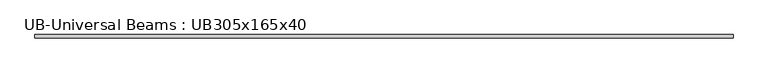
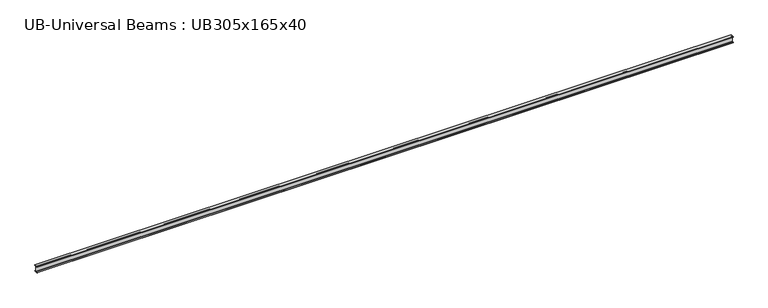
"""IFC4 building model written with IfcOpenShell, lengths in millimetres: beam geometry, UB-Universal Beams : UB305x165x40."""

from ifc_helpers import new_model, si_unit, point, frame, frame_2d, origin, place, context, project, spatial, polyline, circle_curve, trimmed, segment, composite_curve, outline, extrude, source, transform, mapped, element, save


def ub_universal_beams_ub305x165x40_5ea05da3(model_context):
    return source(origin(), model_context, "Body", "SweptSolid", [
        extrude(outline(composite_curve([segment(polyline([(82.5, -141.5), (82.5, -151.7), (-82.5, -151.7), (-82.5, -141.5), (-11.9, -141.5)]), True, "CONTINUOUS"), segment(trimmed(circle_curve(frame_2d((-11.9, -132.6)), 8.9), [point((-11.9, -141.5))], [point((-3.0, -132.6))], True, "CARTESIAN"), True, "CONTINUOUS"), segment(polyline([(-3.0, -132.6), (-3.0, 132.6)]), True, "CONTINUOUS"), segment(trimmed(circle_curve(frame_2d((-11.9, 132.6)), 8.9), [point((-3.0, 132.6))], [point((-11.9, 141.5))], True, "CARTESIAN"), True, "CONTINUOUS"), segment(polyline([(-11.9, 141.5), (-82.5, 141.5), (-82.5, 151.7), (82.5, 151.7), (82.5, 141.5), (11.9, 141.5)]), True, "CONTINUOUS"), segment(trimmed(circle_curve(frame_2d((11.9, 132.6)), 8.9), [point((11.9, 141.5))], [point((3.0, 132.6))], True, "CARTESIAN"), True, "CONTINUOUS"), segment(polyline([(3.0, 132.6), (3.0, -132.6)]), True, "CONTINUOUS"), segment(trimmed(circle_curve(frame_2d((11.9, -132.6)), 8.9), [point((3.0, -132.6))], [point((11.9, -141.5))], True, "CARTESIAN"), True, "CONTINUOUS"), segment(polyline([(11.9, -141.5), (82.5, -141.5)]), True, "CONTINUOUS")], self_intersect=False)), frame((-15953.4, 0.0, 0.0), z_axis=(1.0, 0.0, 0.0), x_axis=(0.0, 1.0, 0.0)), (0.0, 0.0, 1.0), 34323.9),
    ])


if __name__ == "__main__":
    model = new_model("IFC4")
    model_context = context("Model", 3, world=origin())
    ifc_project = project(units=[si_unit("LENGTHUNIT", "METRE", prefix="MILLI")], contexts=[model_context])
    site = spatial("IfcSite", under=ifc_project)
    building = spatial("IfcBuilding", under=site)
    placement = place(None, origin())
    ub_universal_beams_ub305x165x40_shape = ub_universal_beams_ub305x165x40_5ea05da3(model_context)
    element("IfcBeam", 1, ObjectType="UB-Universal Beams : UB305x165x40", at=placement, inside=building, context=model_context, shape_type="MappedRepresentation", body=[
        mapped(ub_universal_beams_ub305x165x40_shape, transform((0.0, 0.0, 0.0), x_axis=(1.0, 0.0, 0.0), y_axis=(0.0, 1.0, 0.0), z_axis=(0.0, 0.0, 1.0))),
    ])
    save(model, "model.ifc")

# Revit data of these elements
# Type "UB-Universal Beams : UB305x165x40"
#   Section Name Key = "UB305X165X40"
#   Width = 16.5 cm
#   Web Thickness = 0.6 cm
#   Web Fillet = 0.89 cm
#   Warping Constant = 164000.0 cm⁶
#   Torsional Moment of Inertia = 14.70 cm⁴
#   Section Area = 51.3 cm²
#   Plastic Modulus weak axis = 142.0 cm³
#   Plastic Modulus strong axis = 623.0 cm³
#   Nominal Weight = 40.2999 kgf/m
#   Moment of Inertia weak axis = 764.00 cm⁴
#   Moment of Inertia strong axis = 8503.00 cm⁴
#   Height = 30.34 cm
#   Flange Thickness = 1.02 cm
#   Elastic Modulus weak axis = 92.6 cm³
#   Elastic Modulus strong axis = 560.0 cm³
#   Centroid Vertical = 15.17 cm
#   Centroid Horizontal = 8.25 cm
#   Bolt Spacing = 9.0 cm
#   Length [instance default] = 1500 mm
#   Structural Material [instance default] = Metal - Steel 43-275
#   Type Comments = ""
#   Assembly Code = ""
# Element 1 (IfcBeam, "UB-Universal Beams : UB305x165x40")
#   Materials on its faces: "Metal - Steel 43-275"
# Materials
#   "Metal - Steel 43-275": class "Metal", colour RGB 247 247 247, transparency 0, Cost = 0
